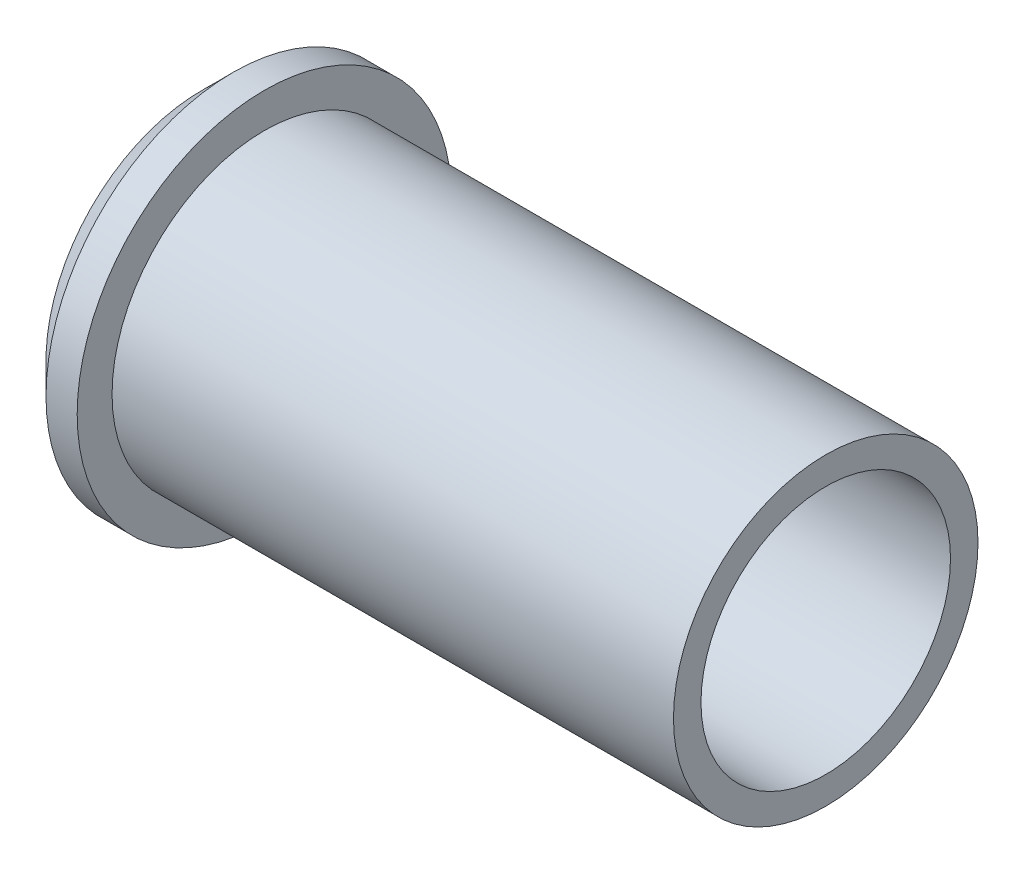
ISO-10303-21;
HEADER;
FILE_DESCRIPTION(('STEP AP214'),'2;1');
FILE_NAME('part.step','',(''),(''),'','','');
FILE_SCHEMA(('AUTOMOTIVE_DESIGN { 1 0 10303 214 1 1 1 1 }'));
ENDSEC;
DATA;
#1=APPLICATION_CONTEXT('core data for automotive mechanical design processes');
#2=APPLICATION_PROTOCOL_DEFINITION('international standard','automotive_design',2000,#1);
#3=PRODUCT_CONTEXT('',#1,'mechanical');
#4=PRODUCT('Part','Part','',(#3));
#5=PRODUCT_RELATED_PRODUCT_CATEGORY('part','',(#4));
#6=PRODUCT_DEFINITION_FORMATION('','',#4);
#7=PRODUCT_DEFINITION_CONTEXT('part definition',#1,'design');
#8=PRODUCT_DEFINITION('design','',#6,#7);
#9=PRODUCT_DEFINITION_SHAPE('','',#8);
#10=(LENGTH_UNIT() NAMED_UNIT(*) SI_UNIT(.MILLI.,.METRE.));
#11=(NAMED_UNIT(*) PLANE_ANGLE_UNIT() SI_UNIT($,.RADIAN.));
#12=(NAMED_UNIT(*) SI_UNIT($,.STERADIAN.) SOLID_ANGLE_UNIT());
#13=UNCERTAINTY_MEASURE_WITH_UNIT(LENGTH_MEASURE(1.E-05),#10,'distance_accuracy_value','');
#14=(GEOMETRIC_REPRESENTATION_CONTEXT(3) GLOBAL_UNCERTAINTY_ASSIGNED_CONTEXT((#13)) GLOBAL_UNIT_ASSIGNED_CONTEXT((#10,
#11,#12)) REPRESENTATION_CONTEXT('',''));
#15=CARTESIAN_POINT('',(0.,0.,0.));
#16=DIRECTION('',(0.,0.,1.));
#17=DIRECTION('',(1.,0.,0.));
#18=AXIS2_PLACEMENT_3D('',#15,#16,#17);
#19=CARTESIAN_POINT('',(15.875,7.74999999999999,0.));
#20=DIRECTION('',(1.,0.,0.));
#21=DIRECTION('',(0.,0.,-1.));
#22=AXIS2_PLACEMENT_3D('',#19,#20,#21);
#23=PLANE('',#22);
#24=CARTESIAN_POINT('',(15.875,0.,0.));
#25=DIRECTION('',(1.,0.,0.));
#26=DIRECTION('',(0.,0.,-1.));
#27=AXIS2_PLACEMENT_3D('',#24,#25,#26);
#28=CIRCLE('',#27,7.74999999999999);
#29=CARTESIAN_POINT('',(15.875,0.,-7.74999999999999));
#30=VERTEX_POINT('',#29);
#31=EDGE_CURVE('E66',#30,#30,#28,.T.);
#32=ORIENTED_EDGE('',*,*,#31,.T.);
#33=EDGE_LOOP('',(#32));
#34=FACE_BOUND('',#33,.T.);
#35=CARTESIAN_POINT('',(15.875,0.,0.));
#36=DIRECTION('',(1.,0.,0.));
#37=DIRECTION('',(0.,0.,-1.));
#38=AXIS2_PLACEMENT_3D('',#35,#36,#37);
#39=CIRCLE('',#38,6.35);
#40=CARTESIAN_POINT('',(15.875,0.,-6.35));
#41=VERTEX_POINT('',#40);
#42=EDGE_CURVE('E51',#41,#41,#39,.T.);
#43=ORIENTED_EDGE('',*,*,#42,.F.);
#44=EDGE_LOOP('',(#43));
#45=FACE_BOUND('',#44,.T.);
#46=ADVANCED_FACE('F39',(#34,#45),#23,.T.);
#47=CARTESIAN_POINT('',(40.7811111111111,0.,0.));
#48=DIRECTION('',(1.,0.,0.));
#49=DIRECTION('',(0.,0.,-1.));
#50=AXIS2_PLACEMENT_3D('',#47,#48,#49);
#51=CYLINDRICAL_SURFACE('',#50,6.34999999999999);
#52=ORIENTED_EDGE('',*,*,#42,.T.);
#53=EDGE_LOOP('',(#52));
#54=FACE_BOUND('',#53,.T.);
#55=CARTESIAN_POINT('',(-15.875,0.,0.));
#56=DIRECTION('',(1.,0.,0.));
#57=DIRECTION('',(0.,0.,-1.));
#58=AXIS2_PLACEMENT_3D('',#55,#56,#57);
#59=CIRCLE('',#58,6.34999999999999);
#60=CARTESIAN_POINT('',(-15.875,0.,-6.34999999999999));
#61=VERTEX_POINT('',#60);
#62=EDGE_CURVE('E54',#61,#61,#59,.T.);
#63=ORIENTED_EDGE('',*,*,#62,.F.);
#64=EDGE_LOOP('',(#63));
#65=FACE_BOUND('',#64,.T.);
#66=ADVANCED_FACE('F87',(#54,#65),#51,.F.);
#67=CARTESIAN_POINT('',(-15.875,8.88999999999999,0.));
#68=DIRECTION('',(-1.,0.,0.));
#69=DIRECTION('',(0.,0.,1.));
#70=AXIS2_PLACEMENT_3D('',#67,#68,#69);
#71=PLANE('',#70);
#72=CARTESIAN_POINT('',(-15.875,0.,0.));
#73=DIRECTION('',(-1.,0.,0.));
#74=DIRECTION('',(0.,0.,1.));
#75=AXIS2_PLACEMENT_3D('',#72,#73,#74);
#76=CIRCLE('',#75,7.93749999999998);
#77=CARTESIAN_POINT('',(-15.875,0.,-7.93749999999998));
#78=VERTEX_POINT('',#77);
#79=EDGE_CURVE('E10',#78,#78,#76,.T.);
#80=ORIENTED_EDGE('',*,*,#79,.T.);
#81=EDGE_LOOP('',(#80));
#82=FACE_BOUND('',#81,.T.);
#83=ORIENTED_EDGE('',*,*,#62,.T.);
#84=EDGE_LOOP('',(#83));
#85=FACE_BOUND('',#84,.T.);
#86=ADVANCED_FACE('F93',(#82,#85),#71,.T.);
#87=CARTESIAN_POINT('',(40.7811111111111,0.,0.));
#88=DIRECTION('',(1.,0.,0.));
#89=DIRECTION('',(0.,0.,-1.));
#90=AXIS2_PLACEMENT_3D('',#87,#88,#89);
#91=CYLINDRICAL_SURFACE('',#90,9.52499999999999);
#92=CARTESIAN_POINT('',(-14.2875,0.,0.));
#93=DIRECTION('',(-1.,0.,0.));
#94=DIRECTION('',(0.,0.,1.));
#95=AXIS2_PLACEMENT_3D('',#92,#93,#94);
#96=CIRCLE('',#95,9.52499999999999);
#97=CARTESIAN_POINT('',(-14.2875,0.,-9.52499999999999));
#98=VERTEX_POINT('',#97);
#99=EDGE_CURVE('E50',#98,#98,#96,.F.);
#100=ORIENTED_EDGE('',*,*,#99,.T.);
#101=EDGE_LOOP('',(#100));
#102=FACE_BOUND('',#101,.T.);
#103=CARTESIAN_POINT('',(-12.7,0.,0.));
#104=DIRECTION('',(1.,0.,0.));
#105=DIRECTION('',(0.,0.,-1.));
#106=AXIS2_PLACEMENT_3D('',#103,#104,#105);
#107=CIRCLE('',#106,9.52499999999999);
#108=CARTESIAN_POINT('',(-12.7,0.,-9.52499999999999));
#109=VERTEX_POINT('',#108);
#110=EDGE_CURVE('E58',#109,#109,#107,.T.);
#111=ORIENTED_EDGE('',*,*,#110,.F.);
#112=EDGE_LOOP('',(#111));
#113=FACE_BOUND('',#112,.T.);
#114=ADVANCED_FACE('F82',(#102,#113),#91,.T.);
#115=CARTESIAN_POINT('',(-12.7,9.52499999999999,0.));
#116=DIRECTION('',(1.,0.,0.));
#117=DIRECTION('',(0.,0.,-1.));
#118=AXIS2_PLACEMENT_3D('',#115,#116,#117);
#119=PLANE('',#118);
#120=ORIENTED_EDGE('',*,*,#110,.T.);
#121=EDGE_LOOP('',(#120));
#122=FACE_BOUND('',#121,.T.);
#123=CARTESIAN_POINT('',(-12.7,0.,0.));
#124=DIRECTION('',(1.,0.,0.));
#125=DIRECTION('',(0.,0.,-1.));
#126=AXIS2_PLACEMENT_3D('',#123,#124,#125);
#127=CIRCLE('',#126,7.74999999999999);
#128=CARTESIAN_POINT('',(-12.7,0.,-7.74999999999999));
#129=VERTEX_POINT('',#128);
#130=EDGE_CURVE('E62',#129,#129,#127,.T.);
#131=ORIENTED_EDGE('',*,*,#130,.F.);
#132=EDGE_LOOP('',(#131));
#133=FACE_BOUND('',#132,.T.);
#134=ADVANCED_FACE('F74',(#122,#133),#119,.T.);
#135=CARTESIAN_POINT('',(40.7811111111111,0.,0.));
#136=DIRECTION('',(1.,0.,0.));
#137=DIRECTION('',(0.,0.,-1.));
#138=AXIS2_PLACEMENT_3D('',#135,#136,#137);
#139=CYLINDRICAL_SURFACE('',#138,7.74999999999999);
#140=ORIENTED_EDGE('',*,*,#130,.T.);
#141=EDGE_LOOP('',(#140));
#142=FACE_BOUND('',#141,.T.);
#143=ORIENTED_EDGE('',*,*,#31,.F.);
#144=EDGE_LOOP('',(#143));
#145=FACE_BOUND('',#144,.T.);
#146=ADVANCED_FACE('F75',(#142,#145),#139,.T.);
#147=CARTESIAN_POINT('',(-14.2875,0.,0.));
#148=DIRECTION('',(1.,0.,0.));
#149=DIRECTION('',(0.,0.,-1.));
#150=AXIS2_PLACEMENT_3D('',#147,#148,#149);
#151=CONICAL_SURFACE('',#150,9.52499999999999,0.78539816339745);
#152=CARTESIAN_POINT('',(-15.875,0.,-7.93749999999998));
#153=CARTESIAN_POINT('',(-15.8584635416667,0.,-7.95403645833331));
#154=CARTESIAN_POINT('',(-15.8419270833333,0.,-7.97057291666665));
#155=CARTESIAN_POINT('',(-15.8088541666667,0.,-8.00364583333332));
#156=CARTESIAN_POINT('',(-15.7923177083333,0.,-8.02018229166665));
#157=CARTESIAN_POINT('',(-15.7592447916667,0.,-8.05325520833332));
#158=CARTESIAN_POINT('',(-15.7427083333333,0.,-8.06979166666665));
#159=CARTESIAN_POINT('',(-15.7096354166667,0.,-8.10286458333331));
#160=CARTESIAN_POINT('',(-15.6930989583333,0.,-8.11940104166665));
#161=CARTESIAN_POINT('',(-15.6600260416667,0.,-8.15247395833332));
#162=CARTESIAN_POINT('',(-15.6434895833333,0.,-8.16901041666665));
#163=CARTESIAN_POINT('',(-15.6104166666667,0.,-8.20208333333332));
#164=CARTESIAN_POINT('',(-15.5938802083333,0.,-8.21861979166665));
#165=CARTESIAN_POINT('',(-15.5608072916667,0.,-8.25169270833332));
#166=CARTESIAN_POINT('',(-15.5442708333333,0.,-8.26822916666665));
#167=CARTESIAN_POINT('',(-15.5111979166667,0.,-8.30130208333332));
#168=CARTESIAN_POINT('',(-15.4946614583333,0.,-8.31783854166665));
#169=CARTESIAN_POINT('',(-15.4615885416667,0.,-8.35091145833332));
#170=CARTESIAN_POINT('',(-15.4450520833333,0.,-8.36744791666665));
#171=CARTESIAN_POINT('',(-15.4119791666667,0.,-8.40052083333332));
#172=CARTESIAN_POINT('',(-15.3954427083333,0.,-8.41705729166665));
#173=CARTESIAN_POINT('',(-15.3623697916667,0.,-8.45013020833332));
#174=CARTESIAN_POINT('',(-15.3458333333333,0.,-8.46666666666665));
#175=CARTESIAN_POINT('',(-15.3127604166667,0.,-8.49973958333332));
#176=CARTESIAN_POINT('',(-15.2962239583333,0.,-8.51627604166665));
#177=CARTESIAN_POINT('',(-15.2631510416667,0.,-8.54934895833332));
#178=CARTESIAN_POINT('',(-15.2466145833333,0.,-8.56588541666665));
#179=CARTESIAN_POINT('',(-15.2135416666667,0.,-8.59895833333332));
#180=CARTESIAN_POINT('',(-15.1970052083333,0.,-8.61549479166665));
#181=CARTESIAN_POINT('',(-15.1639322916667,0.,-8.64856770833332));
#182=CARTESIAN_POINT('',(-15.1473958333333,0.,-8.66510416666665));
#183=CARTESIAN_POINT('',(-15.1143229166667,0.,-8.69817708333332));
#184=CARTESIAN_POINT('',(-15.0977864583333,0.,-8.71471354166665));
#185=CARTESIAN_POINT('',(-15.0647135416667,0.,-8.74778645833332));
#186=CARTESIAN_POINT('',(-15.0481770833333,0.,-8.76432291666665));
#187=CARTESIAN_POINT('',(-15.0151041666667,0.,-8.79739583333332));
#188=CARTESIAN_POINT('',(-14.9985677083333,0.,-8.81393229166665));
#189=CARTESIAN_POINT('',(-14.9654947916667,0.,-8.84700520833332));
#190=CARTESIAN_POINT('',(-14.9489583333333,0.,-8.86354166666665));
#191=CARTESIAN_POINT('',(-14.9158854166667,0.,-8.89661458333332));
#192=CARTESIAN_POINT('',(-14.8993489583333,0.,-8.91315104166665));
#193=CARTESIAN_POINT('',(-14.8662760416667,0.,-8.94622395833332));
#194=CARTESIAN_POINT('',(-14.8497395833333,0.,-8.96276041666665));
#195=CARTESIAN_POINT('',(-14.8166666666667,0.,-8.99583333333332));
#196=CARTESIAN_POINT('',(-14.8001302083333,0.,-9.01236979166666));
#197=CARTESIAN_POINT('',(-14.7670572916667,0.,-9.04544270833332));
#198=CARTESIAN_POINT('',(-14.7505208333333,0.,-9.06197916666666));
#199=CARTESIAN_POINT('',(-14.7174479166667,0.,-9.09505208333332));
#200=CARTESIAN_POINT('',(-14.7009114583333,0.,-9.11158854166666));
#201=CARTESIAN_POINT('',(-14.6678385416667,0.,-9.14466145833332));
#202=CARTESIAN_POINT('',(-14.6513020833333,0.,-9.16119791666666));
#203=CARTESIAN_POINT('',(-14.6182291666667,0.,-9.19427083333332));
#204=CARTESIAN_POINT('',(-14.6016927083333,0.,-9.21080729166666));
#205=CARTESIAN_POINT('',(-14.5686197916667,0.,-9.24388020833332));
#206=CARTESIAN_POINT('',(-14.5520833333333,0.,-9.26041666666666));
#207=CARTESIAN_POINT('',(-14.5190104166667,0.,-9.29348958333332));
#208=CARTESIAN_POINT('',(-14.5024739583333,0.,-9.31002604166666));
#209=CARTESIAN_POINT('',(-14.4694010416667,0.,-9.34309895833333));
#210=CARTESIAN_POINT('',(-14.4528645833333,0.,-9.35963541666666));
#211=CARTESIAN_POINT('',(-14.4197916666667,0.,-9.39270833333333));
#212=CARTESIAN_POINT('',(-14.4032552083333,0.,-9.40924479166666));
#213=CARTESIAN_POINT('',(-14.3701822916667,0.,-9.44231770833333));
#214=CARTESIAN_POINT('',(-14.3536458333333,0.,-9.45885416666666));
#215=CARTESIAN_POINT('',(-14.3205729166667,0.,-9.49192708333333));
#216=CARTESIAN_POINT('',(-14.3040364583333,0.,-9.50846354166666));
#217=CARTESIAN_POINT('',(-14.2875,0.,-9.52499999999999));
#218=B_SPLINE_CURVE_WITH_KNOTS('',3,(#152,#153,#154,#155,#156,#157,#158,#159,#160,#161,#162,
#163,#164,#165,#166,#167,#168,#169,#170,#171,#172,#173,#174,#175,#176,#177,#178,#179,#180,#181,
#182,#183,#184,#185,#186,#187,#188,#189,#190,#191,#192,#193,#194,#195,#196,#197,#198,#199,#200,
#201,#202,#203,#204,#205,#206,#207,#208,#209,#210,#211,#212,#213,#214,#215,#216,#217),
.UNSPECIFIED.,.F.,.F.,(4,2,2,2,2,2,2,2,2,2,2,2,2,2,2,2,2,2,2,2,2,2,2,2,2,2,2,2,2,2,2,2,4),(0.,
0.0701582509458524,0.140316501891705,0.21047475283756,0.280633003783411,0.350791254729263,
0.420949505675118,0.491107756620971,0.561266007566824,0.631424258512678,0.70158250945853,
0.771740760404382,0.841899011350236,0.91205726229609,0.982215513241942,1.0523737641878,
1.12253201513365,1.1926902660795,1.26284851702535,1.33300676797121,1.40316501891706,
1.47332326986291,1.54348152080877,1.61363977175462,1.68379802270047,1.75395627364633,
1.82411452459218,1.89427277553803,1.96443102648389,2.03458927742974,2.10474752837559,
2.17490577932145,2.2450640302673),.UNSPECIFIED.);
#219=EDGE_CURVE('BSEAM45',#78,#98,#218,.T.);
#220=ORIENTED_EDGE('',*,*,#79,.F.);
#221=ORIENTED_EDGE('',*,*,#99,.F.);
#222=ORIENTED_EDGE('',*,*,#219,.T.);
#223=ORIENTED_EDGE('',*,*,#219,.F.);
#224=EDGE_LOOP('',(#220,#222,#221,#223));
#225=FACE_BOUND('',#224,.T.);
#226=ADVANCED_FACE('F45',(#225),#151,.T.);
#227=CLOSED_SHELL('',(#46,#66,#86,#114,#134,#146,#226));
#228=MANIFOLD_SOLID_BREP('B2',#227);
#229=ADVANCED_BREP_SHAPE_REPRESENTATION('',(#18,#228),#14);
#230=SHAPE_DEFINITION_REPRESENTATION(#9,#229);
ENDSEC;
END-ISO-10303-21;
